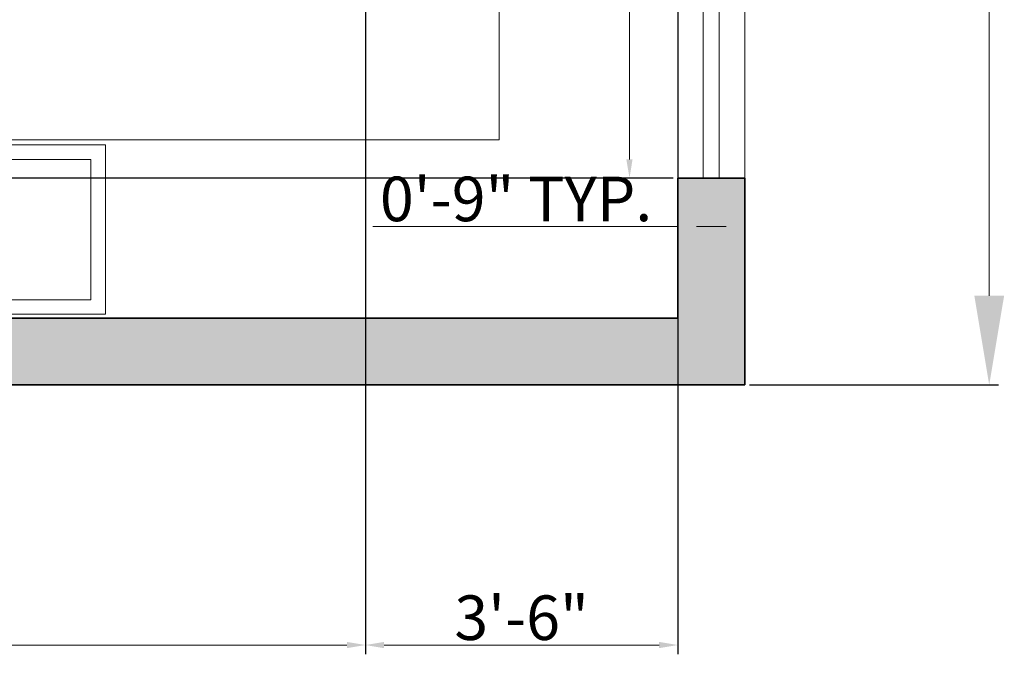
# Model space of a CAD drawing. Units: inches. Extents: x 2696 to 3240, y 1564 to 2310.
# Tile 26 of 76: x 3102 to 3235, y 1569 to 1654. Entities that reach past the tile are written whole.
import ezdxf

# ---------------------------------------------------------------- set-up
doc = ezdxf.new("R2010")
doc.units = ezdxf.units.IN
for name, color, linetype, lineweight in [('A-ANNO-DIMS', 3, 'Continuous', 18), ('A-FLOR-CASE', 8, 'Continuous', 18), ('A-FLOR-FIXT', 8, 'Continuous', 18), ('A-WALL', 7, 'Continuous', 35), ('A-WALL-PATT', 9, 'Continuous', 13), ('WINDOW', 2, 'Continuous', 18)]:
    doc.layers.add(name, color=color, linetype=linetype, lineweight=lineweight)
doc.styles.add('TIMES NEW', font='times.ttf')
doc.dimstyles.new('Siddhuu', dxfattribs={"dimtxt": 6, "dimasz": 2.5, "dimexe": 1.25, "dimexo": 0.625, "dimtad": 1, "dimdec": 1, "dimlunit": 4, "dimtxsty": 'TIMES NEW', "dimcen": 2.5, "dimclrd": 256, "dimclre": 1, "dimclrt": 7, "dimadec": 0, "dimazin": 0, "dimtfac": 1, "dimtdec": 1, "dimtmove": 0, "dimatfit": 3, "dimfxl": 1, "dimtolj": 1, "dimlwd": -1, "dimarcsym": 0})

# ---------------------------------------------------------------- blocks, each defined once
blk = doc.blocks.new('WD_WIN4')
for p, q in [((-0.5, 0.5), (0.5, 0.5)), ((-0.5, 0.12), (0.5, 0.12)), ((-0.5, -0.12), (0.5, -0.12)), ((-0.5, -0.5), (0.5, -0.5))]:
    blk.add_line(p, q)
blk = doc.blocks.new('*D10')
at = {"layer": 'A-ANNO-DIMS', "color": 0, "lineweight": -2, "transparency": 16777216}
for p, q in [((3200.24, 2262.2), (3233.75, 2262.2)), ((3200.24, 1605.2), (3233.75, 1605.2))]:
    blk.add_line(p, q, dxfattribs=at)
at = {"layer": 'A-ANNO-DIMS', "color": 0, "transparency": 16777216}
blk.add_line((3232.5, 2250.2), (3232.5, 1617.2), dxfattribs=at)
for points in [[(3230.5, 2250.2), (3234.5, 2250.2), (3232.5, 2262.2)], [(3230.5, 1617.2), (3234.5, 1617.2), (3232.5, 1605.2)]]:
    blk.add_solid(points, dxfattribs=at)
at = {"layer": 'Defpoints', "color": 0, "transparency": 16777216}
for p in [(3199.61, 2262.2), (3199.61, 1605.2), (3232.5, 1605.2)]:
    blk.add_point(p, dxfattribs=at)
at = {"layer": 'A-ANNO-DIMS', "color": 0, "transparency": 16777216, "insert": (3222.71, 1933.7), "char_height": 18, "attachment_point": 5, "rotation": 90, "style": 'TIMES NEW'}
blk.add_mtext("\\A1;54'", dxfattribs=at)
blk = doc.blocks.new('SINK-KITCHEN')
for points in [[(0, 22.8), (31.04, 22.8), (31.04, 0), (0, 0)], [(1.97, 20.82), (29.07, 20.82), (29.07, 1.97), (1.97, 1.97)]]:
    blk.add_lwpolyline(points, close=True)
blk.add_circle((15.52, 11.4), 1.71)
blk = doc.blocks.new('*D26')
at = {"layer": 'A-ANNO-DIMS', "transparency": 16777216}
for p, q in [((3184.12, 1676.35), (3184.12, 1772.17)), ((3184.12, 1635.55), (3184.12, 1673.85))]:
    blk.add_line(p, q, dxfattribs=at)
at = {"layer": 'A-ANNO-DIMS', "color": 1, "lineweight": -2, "transparency": 16777216}
for p, q in [((3189.99, 1676.35), (3182.87, 1676.35)), ((3189.99, 1633.05), (3182.87, 1633.05))]:
    blk.add_line(p, q, dxfattribs=at)
at = {"layer": 'A-ANNO-DIMS', "transparency": 16777216}
for points in [[(3183.7, 1673.85), (3184.53, 1673.85), (3184.12, 1676.35)], [(3183.7, 1635.55), (3184.53, 1635.55), (3184.12, 1633.05)]]:
    blk.add_solid(points, dxfattribs=at)
at = {"layer": 'Defpoints', "color": 0, "transparency": 16777216}
for p in [(3184.12, 1676.35), (3190.61, 1676.35), (3190.61, 1633.05)]:
    blk.add_point(p, dxfattribs=at)
at = {"layer": 'A-ANNO-DIMS', "color": 7, "transparency": 16777216, "insert": (3180.35, 1725.51), "char_height": 6, "attachment_point": 5, "rotation": 90, "style": 'TIMES NEW'}
blk.add_mtext('\\A1;WINDOW 3\'-7 1/2" TYP.', dxfattribs=at)
blk = doc.blocks.new('*D27')
at = {"layer": 'A-ANNO-DIMS', "color": 1, "lineweight": -2, "transparency": 16777216}
for p, q in [((3190.61, 1632.42), (3190.61, 1625.3)), ((3199.61, 1632.42), (3199.61, 1625.3))]:
    blk.add_line(p, q, dxfattribs=at)
at = {"layer": 'A-ANNO-DIMS', "transparency": 16777216}
for p, q in [((3190.61, 1626.55), (3149.62, 1626.55)), ((3197.11, 1626.55), (3193.11, 1626.55))]:
    blk.add_line(p, q, dxfattribs=at)
for points in [[(3193.11, 1626.97), (3193.11, 1626.13), (3190.61, 1626.55)], [(3197.11, 1626.97), (3197.11, 1626.13), (3199.61, 1626.55)]]:
    blk.add_solid(points, dxfattribs=at)
at = {"layer": 'Defpoints', "color": 0, "transparency": 16777216}
for p in [(3190.61, 1633.05), (3199.61, 1633.05), (3190.61, 1626.55)]:
    blk.add_point(p, dxfattribs=at)
at = {"layer": 'A-ANNO-DIMS', "color": 7, "transparency": 16777216, "insert": (3168.87, 1630.24), "char_height": 6, "attachment_point": 5, "style": 'TIMES NEW'}
blk.add_mtext('\\A1;0\'-9" TYP.', dxfattribs=at)
blk = doc.blocks.new('*D51')
at = {"layer": 'A-ANNO-DIMS', "color": 1, "lineweight": -2, "transparency": 16777216}
for p, q in [((3016.61, 1979.58), (3016.61, 1568.95)), ((3148.61, 1979.58), (3148.61, 1568.95))]:
    blk.add_line(p, q, dxfattribs=at)
at = {"layer": 'A-ANNO-DIMS', "transparency": 16777216}
blk.add_line((3019.11, 1570.2), (3146.11, 1570.2), dxfattribs=at)
for points in [[(3019.11, 1570.62), (3019.11, 1569.78), (3016.61, 1570.2)], [(3146.11, 1570.62), (3146.11, 1569.78), (3148.61, 1570.2)]]:
    blk.add_solid(points, dxfattribs=at)
at = {"layer": 'Defpoints', "color": 0, "transparency": 16777216}
for p in [(3016.61, 1980.2), (3148.61, 1980.2), (3148.61, 1570.2)]:
    blk.add_point(p, dxfattribs=at)
at = {"layer": 'A-ANNO-DIMS', "color": 7, "transparency": 16777216, "insert": (3082.61, 1573.88), "char_height": 6, "attachment_point": 5, "style": 'TIMES NEW'}
blk.add_mtext('\\A1;11\'-0"', dxfattribs=at)
blk = doc.blocks.new('*D52')
at = {"layer": 'A-ANNO-DIMS', "color": 1, "lineweight": -2, "transparency": 16777216}
for p, q in [((3148.61, 1979.58), (3148.61, 1568.95)), ((3190.61, 1979.58), (3190.61, 1568.95))]:
    blk.add_line(p, q, dxfattribs=at)
at = {"layer": 'A-ANNO-DIMS', "transparency": 16777216}
blk.add_line((3151.11, 1570.2), (3188.11, 1570.2), dxfattribs=at)
for points in [[(3151.11, 1570.62), (3151.11, 1569.78), (3148.61, 1570.2)], [(3188.11, 1570.62), (3188.11, 1569.78), (3190.61, 1570.2)]]:
    blk.add_solid(points, dxfattribs=at)
at = {"layer": 'Defpoints', "color": 0, "transparency": 16777216}
for p in [(3148.61, 1980.2), (3190.61, 1980.2), (3190.61, 1570.2)]:
    blk.add_point(p, dxfattribs=at)
at = {"layer": 'A-ANNO-DIMS', "color": 7, "transparency": 16777216, "insert": (3169.61, 1573.88), "char_height": 6, "attachment_point": 5, "style": 'TIMES NEW'}
blk.add_mtext('\\A1;3\'-6"', dxfattribs=at)
blk = doc.blocks.new('*D81')
at = {"layer": 'A-ANNO-DIMS', "color": 1, "lineweight": -2, "transparency": 16777216}
for p, q in [((3189.99, 1633.05), (2709.36, 1633.05)), ((3189.99, 1614.2), (2709.36, 1614.2))]:
    blk.add_line(p, q, dxfattribs=at)
at = {"layer": 'A-ANNO-DIMS', "transparency": 16777216}
blk.add_line((2710.61, 1616.7), (2710.61, 1630.55), dxfattribs=at)
for points in [[(2710.19, 1630.55), (2711.03, 1630.55), (2710.61, 1633.05)], [(2710.19, 1616.7), (2711.03, 1616.7), (2710.61, 1614.2)]]:
    blk.add_solid(points, dxfattribs=at)
at = {"layer": 'Defpoints', "color": 0, "transparency": 16777216}
for p in [(2710.61, 1633.05), (3190.61, 1633.05), (3190.61, 1614.2)]:
    blk.add_point(p, dxfattribs=at)
at = {"layer": 'A-ANNO-DIMS', "color": 7, "transparency": 16777216, "insert": (2706.93, 1623.62), "char_height": 6, "attachment_point": 5, "rotation": 90, "style": 'TIMES NEW'}
blk.add_mtext('\\A1;1\'-7"', dxfattribs=at)

msp = doc.modelspace()

# ---------------------------------------------------------------- hatches: boundary and pattern name
at = {"layer": 'A-WALL-PATT', "transparency": 33554556}
h = msp.add_hatch(color=256, dxfattribs=at)
h.dxf.hatch_style = 1
h.paths.add_polyline_path([(2879.11, 2253.2), (2905.91, 2253.2), (2905.91, 2262.2), (2841.89, 2262.2), (2841.89, 2253.2), (2870.11, 2253.2), (2870.11, 2176.6), (2965.71, 2176.6), (2965.71, 2206.7), (2973.58, 2206.7), (2973.58, 2215.7), (2965.71, 2215.7), (2965.71, 2262.2), (2929.91, 2262.2), (2929.91, 2253.2), (2956.71, 2253.2), (2956.71, 2185.6), (2879.11, 2185.6)])
h.paths.add_polyline_path([(2782.83, 2262.2), (2745.61, 2262.2), (2745.61, 2228.73), (2754.61, 2228.73), (2754.61, 2253.2), (2782.83, 2253.2)])
h.paths.add_polyline_path([(2754.61, 2136.2), (2965.71, 2136.2), (2965.71, 2145.2), (2879.11, 2145.2), (2879.11, 2147.07), (2877.34, 2147.07), (2870.11, 2147.07), (2870.11, 2145.2), (2754.61, 2145.2), (2754.61, 2169.67), (2745.61, 2169.67), (2745.61, 2000.2), (2754.61, 2000.2), (2754.61, 2019.2), (2849.08, 2019.2), (2849.08, 2023.7), (2841.21, 2023.7), (2841.21, 2051.83), (2836.71, 2051.83), (2836.71, 2023.7), (2754.61, 2023.7), (2754.61, 2091.2), (2836.71, 2091.2), (2836.71, 2087.83), (2841.21, 2087.83), (2841.21, 2095.7), (2754.61, 2095.7)])
h.paths.add_polyline_path([(2965.71, 2136.2), (2956.71, 2136.2), (2956.71, 2023.7), (2885.08, 2023.7), (2885.08, 2019.2), (2956.71, 2019.2), (2956.71, 1950.58), (2965.71, 1950.58), (2965.71, 1980.2), (2973.58, 1980.2), (2973.58, 1989.2), (2965.71, 1989.2)])
h.paths.add_polyline_path([(2754.61, 1906.7), (2880.21, 1906.7), (2884.71, 1906.7), (2956.71, 1906.7), (2956.71, 1792.7), (2944.71, 1792.7), (2944.71, 1783.7), (2956.71, 1783.7), (2956.71, 1740.2), (2884.71, 1740.2), (2884.71, 1783.7), (2896.71, 1783.7), (2896.71, 1792.7), (2884.71, 1792.7), (2884.71, 1846.7), (2880.21, 1846.7), (2880.21, 1740.2), (2754.61, 1740.2), (2754.61, 1777.2), (2745.61, 1777.2), (2745.61, 1692.7), (2754.61, 1692.7), (2754.61, 1731.2), (2956.71, 1731.2), (2956.71, 1723.33), (2965.71, 1723.33), (2965.71, 1884.2), (2973.58, 1884.2), (2973.58, 1893.2), (2965.71, 1893.2), (2965.71, 1914.58), (2956.71, 1914.58), (2956.71, 1911.2), (2754.61, 1911.2), (2754.61, 1930.2), (2745.61, 1930.2), (2745.61, 1817.2), (2754.61, 1817.2), (2754.61, 1854.2), (2826.61, 1854.2), (2826.61, 1868.83), (2822.11, 1868.83), (2822.11, 1858.7), (2754.61, 1858.7)])
h.paths.add_polyline_path([(2965.71, 1656.2), (3008.24, 1656.2), (3008.24, 1665.2), (2965.71, 1665.2), (2965.71, 1693.33), (2956.71, 1693.33), (2956.71, 1686.2), (2934.58, 1686.2), (2934.58, 1681.7), (2956.71, 1681.7), (2956.71, 1614.2), (2896.71, 1614.2), (2896.71, 1681.7), (2904.58, 1681.7), (2904.58, 1686.2), (2892.21, 1686.2), (2892.21, 1614.2), (2858.41, 1614.2), (2858.41, 1605.2), (2965.71, 1605.2)])
h.paths.add_polyline_path([(2788.41, 1614.2), (2754.61, 1614.2), (2754.61, 1652.7), (2745.61, 1652.7), (2745.61, 1605.2), (2788.41, 1605.2)])
h.paths.add_polyline_path([(3199.61, 1633.05), (3190.61, 1633.05), (3190.61, 1614.2), (3082.61, 1614.2), (3082.61, 1665.2), (3070.24, 1665.2), (3070.24, 1656.2), (3078.11, 1656.2), (3078.11, 1605.2), (3199.61, 1605.2)])
h.paths.add_polyline_path([(3199.61, 1702.05), (3190.61, 1702.05), (3190.61, 1699.7), (3106.61, 1699.7), (3106.61, 1747.7), (3190.61, 1747.7), (3190.61, 1752.2), (3082.61, 1752.2), (3082.61, 1760.08), (3078.11, 1760.08), (3078.11, 1747.7), (3102.11, 1747.7), (3102.11, 1699.7), (3078.11, 1699.7), (3078.11, 1695.2), (3190.61, 1695.2), (3190.61, 1676.35), (3199.61, 1676.35)])
h.paths.add_polyline_path([(3199.61, 1783.2), (3190.61, 1783.2), (3190.61, 1745.35), (3199.61, 1745.35)])
h.paths.add_polyline_path([(3082.61, 1884.2), (3190.61, 1884.2), (3190.61, 1853.2), (3199.61, 1853.2), (3199.61, 1901.7), (3190.61, 1901.7), (3190.61, 1893.2), (3005.58, 1893.2), (3005.58, 1891.28), (3005.58, 1884.2), (3078.11, 1884.2), (3078.11, 1792.08), (3082.61, 1792.08)])
h.paths.add_polyline_path([(3199.61, 1994.7), (3190.61, 1994.7), (3190.61, 1989.2), (3073.71, 1989.2), (3073.71, 2034.2), (3069.21, 2034.2), (3069.21, 1989.2), (3005.58, 1989.2), (3005.58, 1980.2), (3190.61, 1980.2), (3190.61, 1971.7), (3199.61, 1971.7)])
h.paths.add_polyline_path([(3199.61, 2155.2), (3190.61, 2155.2), (3190.61, 2064.7), (3199.61, 2064.7)])
h.paths.add_polyline_path([(3190.61, 2074.7), (3106.61, 2074.7), (3106.61, 2122.7), (3190.61, 2122.7), (3190.61, 2127.2), (3082.71, 2127.2), (3082.71, 2135.08), (3073.71, 2135.08), (3073.71, 2122.7), (3102.11, 2122.7), (3102.11, 2074.7), (3069.21, 2074.7), (3069.21, 2070.2), (3190.61, 2070.2)])
h.paths.add_polyline_path([(3082.71, 2253.2), (3190.61, 2253.2), (3190.61, 2225.2), (3199.61, 2225.2), (3199.61, 2262.2), (3073.71, 2262.2), (3073.71, 2215.7), (3035.58, 2215.7), (3035.58, 2206.7), (3073.71, 2206.7), (3073.71, 2171.08), (3082.71, 2171.08)])

# ---------------------------------------------------------------- linework, layer by layer
at = {"layer": 'A-FLOR-CASE'}
for p, q in [((3166.61, 1638.2), (3166.61, 1695.2)), ((3082.61, 1638.2), (3166.61, 1638.2))]:
    msp.add_line(p, q, dxfattribs=at)
at = {"layer": 'A-WALL'}
for p, q in [((3190.61, 1614.2), (3190.61, 1633.05)), ((3190.61, 1633.05), (3199.61, 1633.05)), ((3199.61, 1605.2), (3199.61, 1633.05)), ((3082.61, 1614.2), (3190.61, 1614.2)), ((3078.11, 1605.2), (3199.61, 1605.2))]:
    msp.add_line(p, q, dxfattribs=at)

# ---------------------------------------------------------------- block references
at = {"layer": 'A-FLOR-FIXT'}
msp.add_blockref('SINK-KITCHEN', (3082.61, 1614.71), dxfattribs=at)
at = {"layer": 'WINDOW', "xscale": 43.30708661417323, "yscale": 8.999999999999545, "zscale": 43.30708661417323, "rotation": 90}
msp.add_blockref('WD_WIN4', (3195.11, 1654.7), dxfattribs=at)

# ---------------------------------------------------------------- dimensions: what is measured, and where the dimension line sits
at = {"layer": 'A-ANNO-DIMS'}
for base, p1, p2, angle, text, override, picture, middle in [((3232.5, 1605.2), (3199.61, 2262.2), (3199.61, 1605.2), 90, "54'", {"dimtxt": 18, "dimasz": 12, "dimclrd": 0, "dimclre": 0, "dimclrt": 0}, '*D10', (3222.71, 1933.7)), ((3184.12, 1676.35), (3190.61, 1633.05), (3190.61, 1676.35), 90, 'WINDOW <> TYP.', {"dimdec": 1, "dimlfac": 1, "dimrnd": 0, "dimzin": 1, "dimdsep": 46, "dimlunit": 4, "dimfrac": 2}, '*D26', (3180.35, 1725.51)), ((3190.61, 1626.55), (3199.61, 1633.05), (3190.61, 1633.05), 180, '<> TYP.', {"dimdec": 1, "dimlfac": 1, "dimrnd": 0, "dimzin": 1, "dimdsep": 46, "dimlunit": 4, "dimfrac": 2}, '*D27', (3168.87, 1630.24))]:
    dim = msp.add_linear_dim(base=base, p1=p1, p2=p2, angle=angle, text=text, dimstyle='Siddhuu', override=override, dxfattribs=at)
    dim.commit()
    dim.dimension.update_dxf_attribs({"geometry": picture, "text_midpoint": middle})
for base, p1, p2, picture, middle in [((3148.61, 1570.2), (3016.61, 1980.2), (3148.61, 1980.2), '*D51', (3082.61, 1573.88)), ((3190.61, 1570.2), (3148.61, 1980.2), (3190.61, 1980.2), '*D52', (3169.61, 1573.88))]:
    dim = msp.add_linear_dim(base=base, p1=p1, p2=p2, dimstyle='Siddhuu', override={"dimdec": 1, "dimlfac": 1, "dimrnd": 0, "dimzin": 1, "dimdsep": 46, "dimlunit": 4, "dimfrac": 2}, dxfattribs=at)
    dim.commit()
    dim.dimension.update_dxf_attribs({"geometry": picture, "text_midpoint": middle})
dim = msp.add_linear_dim(base=(2710.6114, 1633.0476), p1=(3190.6114, 1614.2011), p2=(3190.6114, 1633.0476), angle=90, dimstyle='Siddhuu', override={"dimdec": 1, "dimlfac": 1, "dimrnd": 0, "dimzin": 1, "dimdsep": 46, "dimlunit": 4, "dimfrac": 2}, dxfattribs=at)
dim.commit()
dim.dimension.update_dxf_attribs({"geometry": '*D81', "text_midpoint": (2706.9258, 1623.6243)})

doc.saveas('drawing.dxf')
